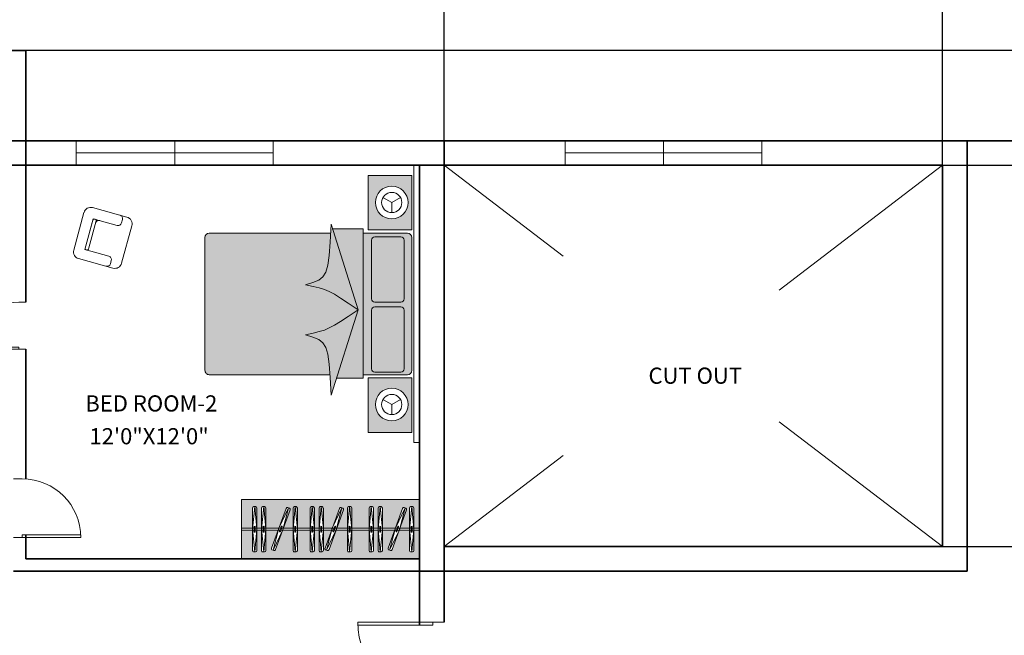
# Model space of a CAD drawing. Units: millimetres. Extents: x 27017497 to 27018854, y 7058029 to 7059154.
# Tile 60 of 91: x 27017886 to 27018246, y 7058409 to 7058634. Entities that reach past the tile are written whole.
import ezdxf

# ---------------------------------------------------------------- set-up
doc = ezdxf.new("R2010")
doc.units = ezdxf.units.MM
for name, color, linetype, lineweight in [('A-ANNO-DIMS', 2, 'Continuous', 18), ('A-AREA-IDEN', 7, 'Continuous', 18), ('A-DOOR', 4, 'Continuous', 20), ('A-FLOR-CASE', 8, 'Continuous', 20), ('A-FLOR-CASE-PATT', 44, 'Continuous', 13), ('A-FLOR-OPEN', 9, 'Continuous', 13), ('A-FURN', 8, 'Continuous', 18), ('A-GLAZ', 4, 'Continuous', 18), ('A-WALL', 7, 'Continuous', 35)]:
    doc.layers.add(name, color=color, linetype=linetype, lineweight=lineweight)
doc.layers.add('A-FURN-PATT', color=177, linetype='Continuous', lineweight=13, true_color=0x293189)
doc.styles.get("Standard").update_dxf_attribs({"font": 'arial.ttf'})
doc.dimstyles.get("Standard").update_dxf_attribs({"dimtxt": 0.18, "dimasz": 0.18, "dimexe": 0.18, "dimexo": 0.0625, "dimgap": 0.09, "dimtad": 0, "dimtih": 1, "dimtoh": 1, "dimdec": 4, "dimzin": 0, "dimdsep": 46, "dimtxsty": 'Standard', "dimcen": 0.09, "dimadec": 0, "dimazin": 0, "dimtfac": 1, "dimtdec": 4, "dimtofl": 0, "dimtmove": 0, "dimatfit": 3, "dimfxl": 1, "dimtolj": 1, "dimtzin": 0, "dimarcsym": 0})

# ---------------------------------------------------------------- blocks, each defined once
blk = doc.blocks.new('CAMMAT')
for p, q in [((1.2731, 0), (-1.2731, 0)), ((1.2731, 0), (1.2731, -0.05)), ((-1.2731, 0), (-1.2731, -0.05)), ((1.2731, -0.05), (-1.2731, -0.05)), ((-1.18, -0.07), (-1.18, -0.47)), ((-1.18, -0.07), (-0.68, -0.07)), ((-0.68, -0.07), (-0.68, -0.47)), ((0.61, -0.07), (-0.61, -0.07)), ((0.68, -0.07), (0.68, -0.47)), ((0.68, -0.07), (1.18, -0.07)), ((1.18, -0.07), (1.18, -0.47)), ((-0.931, -0.2541), (-0.9775, -0.1737)), ((-0.65, -0.11), (-0.65, -0.5169)), ((-0.6152, -0.1695), (-0.6152, -0.4095)), ((-0.0465, -0.1395), (-0.5852, -0.1395)), ((-0.0165, -0.1695), (-0.0165, -0.4095)), ((0.0274, -0.1695), (0.0274, -0.4095)), ((0.5962, -0.1395), (0.0574, -0.1395)), ((0.6262, -0.1695), (0.6262, -0.4095)), ((0.65, -0.11), (0.65, -0.5169)), ((0.9242, -0.2541), (0.8777, -0.1737)), ((-0.931, -0.2541), (-0.9775, -0.3346)), ((-0.931, -0.2541), (-0.8381, -0.2541)), ((0.9242, -0.2541), (0.8777, -0.3346)), ((0.9242, -0.2541), (1.0171, -0.2541)), ((-0.0465, -0.4395), (-0.5852, -0.4395)), ((0.5962, -0.4395), (0.0574, -0.4395)), ((-1.18, -0.47), (-0.68, -0.47)), ((-0.6904, -0.5169), (-0.6904, -0.8)), ((-0.6904, -0.5169), (0.6826, -0.5169)), ((0.68, -0.47), (1.18, -0.47)), ((0.6826, -0.5169), (0.6826, -0.7603)), ((0.0535, -0.5623), (-0.7312, -0.8093)), ((0.0535, -0.5623), (0.8382, -0.8093)), ((-0.65, -0.8139), (-0.65, -1.93)), ((0.65, -0.8204), (0.65, -1.93)), ((0.61, -1.97), (-0.61, -1.97))]:
    blk.add_line(p, q)
for points in [[(-0.1761, -1.0476), (-0.161, -0.9772), (-0.1474, -0.921), (-0.1326, -0.8732), (-0.1139, -0.8282), (-0.0886, -0.7803), (-0.0541, -0.7238), (-0.0076, -0.653), (0.0535, -0.5623)], [(0.2832, -1.0476), (0.2681, -0.9772), (0.2545, -0.921), (0.2396, -0.8732), (0.2209, -0.8282), (0.1957, -0.7803), (0.1611, -0.7238), (0.1147, -0.653), (0.0535, -0.5623)], [(-0.7312, -0.8093), (-0.5683, -0.8185), (-0.4451, -0.828), (-0.3552, -0.8406), (-0.2919, -0.8591), (-0.2489, -0.8862), (-0.2196, -0.9248), (-0.1975, -0.9777), (-0.1761, -1.0476)], [(0.8382, -0.8093), (0.6753, -0.8185), (0.5522, -0.828), (0.4622, -0.8406), (0.399, -0.8591), (0.356, -0.8862), (0.3267, -0.9248), (0.3046, -0.9777), (0.2832, -1.0476)]]:
    blk.add_lwpolyline(points)
for centre, radius in [((-0.931, -0.2541), 0.15), ((-0.931, -0.2541), 0.0929), ((0.9242, -0.2541), 0.15), ((0.9242, -0.2541), 0.0929)]:
    blk.add_circle(centre, radius)
for centre, radius, start, end in [((-0.61, -0.11), 0.04, 90, 180), ((0.61, -0.11), 0.04, 0, 90), ((-0.5852, -0.1695), 0.03, 90, 180), ((-0.0465, -0.1695), 0.03, 360, 90), ((0.0574, -0.1695), 0.03, 90, 180), ((0.5962, -0.1695), 0.03, 360, 90), ((-0.5852, -0.4095), 0.03, 180, 270), ((-0.0465, -0.4095), 0.03, 270, 360), ((0.0574, -0.4095), 0.03, 180, 270), ((0.5962, -0.4095), 0.03, 270, 360), ((-0.61, -1.93), 0.04, 180, 270), ((0.61, -1.93), 0.04, 270, 360)]:
    blk.add_arc(centre, radius, start, end)
blk = doc.blocks.new('*U2')
for p, q in [((0, 0), (0, -6)), ((40, 0), (40, -6))]:
    blk.add_line(p, q)
blk.add_lwpolyline([(0, 0), (0, 40), (1.75, 40), (1.75, 0)], close=True)
blk.add_arc((0, 0), 40, 0, 90)
blk = doc.blocks.new('CHAIR-OCCASIONAL')
for p, q in [((19.6, 18.74), (7.02, 22.21)), ((3.87, 20.42), (0.09, 6.71)), ((4.13, 6.92), (7.23, 18.17)), ((5.25, 10.97), (7.23, 18.17)), ((16.06, 15.73), (7.23, 18.17)), ((7.23, 18.17), (16.06, 15.73)), ((7.23, 18.17), (16.06, 15.73)), ((7.73, 18.03), (7.97, 17.97)), ((7.73, 18.03), (7.97, 17.97)), ((5.25, 10.97), (7.1, 17.68)), ((8.33, 17.34), (5.63, 7.52)), ((17.6, 1.88), (21.39, 15.6)), ((17.64, 16.63), (17.98, 17.86)), ((17.64, 16.63), (17.98, 17.86)), ((5.63, 7.52), (5.5, 7.07)), ((12.96, 4.48), (4.13, 6.92)), ((4.87, 6.71), (4.63, 6.78)), ((1.88, 3.56), (14.46, 0.09)), ((13.86, 2.91), (13.52, 1.68))]:
    blk.add_line(p, q)
for centre, radius, start, end in [((6.34, 19.74), 2.56, 74.5879, 164.5879), ((7.59, 17.54), 0.512, 74.5879, 164.5879), ((16.74, 18.2), 1.28, 344.5879, 74.5879), ((16.74, 18.2), 1.28, 344.5879, 74.5879), ((18.92, 16.28), 2.56, 344.5879, 74.5879), ((7.84, 17.47), 0.512, 344.5879, 74.5879), ((9.36, 16.26), 1.28, 74.5879, 164.5879), ((16.4, 16.97), 1.28, 254.5879, 344.5879), ((16.4, 16.97), 1.28, 254.5879, 344.5879), ((4.76, 7.28), 0.512, 164.5879, 254.5879), ((2.56, 6.03), 2.56, 164.5879, 254.5879), ((5.01, 7.21), 0.512, 254.5879, 344.5879), ((12.62, 3.25), 1.28, 344.5879, 74.5879), ((12.28, 2.02), 1.28, 254.5879, 344.5879), ((15.14, 2.56), 2.56, 254.5879, 344.5879)]:
    blk.add_arc(centre, radius, start, end)
blk = doc.blocks.new('WARDROBE-HANGING')
for p, q in [((0, 21.74), (65.21, 21.74)), ((0, 0), (0, 21.74)), ((65.21, 0), (65.21, 21.74)), ((4.86, 19.15), (4.08, 10.88)), ((4.08, 18.62), (4.08, 3.13)), ((5.18, 19.15), (4.55, 19.15)), ((4.86, 19.15), (5.64, 10.88)), ((5.64, 18.62), (5.64, 3.13)), ((8.14, 19.15), (7.35, 10.88)), ((7.35, 18.62), (7.35, 3.13)), ((8.45, 19.15), (7.82, 19.15)), ((8.14, 19.15), (8.92, 10.88)), ((8.92, 18.62), (8.92, 3.13)), ((16.33, 18.5), (11.03, 3.94)), ((17.25, 18.73), (13.68, 11.22)), ((17.25, 18.73), (15.15, 10.68)), ((17.54, 18.62), (16.95, 18.83)), ((19.66, 19.15), (18.88, 10.88)), ((18.88, 18.62), (18.88, 3.13)), ((19.98, 19.15), (19.35, 19.15)), ((19.66, 19.15), (20.45, 10.88)), ((20.45, 18.62), (20.45, 3.13)), ((25.9, 19.15), (25.12, 10.88)), ((25.12, 18.62), (25.12, 3.13)), ((26.21, 19.15), (25.59, 19.15)), ((25.9, 19.15), (26.68, 10.88)), ((26.68, 18.62), (26.68, 3.13)), ((29.17, 19.15), (28.39, 10.88)), ((28.39, 18.62), (28.39, 3.13)), ((29.49, 19.15), (28.86, 19.15)), ((29.17, 19.15), (29.96, 10.88)), ((29.96, 18.62), (29.96, 3.13)), ((35.87, 18.5), (30.57, 3.94)), ((36.78, 18.73), (33.22, 11.22)), ((36.78, 18.73), (34.69, 10.68)), ((37.08, 18.62), (36.49, 18.83)), ((39.59, 19.15), (38.81, 10.88)), ((38.81, 18.62), (38.81, 3.13)), ((39.9, 19.15), (39.28, 19.15)), ((39.59, 19.15), (40.37, 10.88)), ((40.37, 18.62), (40.37, 3.13)), ((47.49, 19.15), (46.71, 10.88)), ((46.71, 18.62), (46.71, 3.13)), ((47.81, 19.15), (47.18, 19.15)), ((47.49, 19.15), (48.28, 10.88)), ((48.28, 18.62), (48.28, 3.13)), ((50.77, 19.15), (49.98, 10.88)), ((49.98, 18.62), (49.98, 3.13)), ((51.08, 19.15), (50.45, 19.15)), ((50.77, 19.15), (51.55, 10.88)), ((51.55, 18.62), (51.55, 3.13)), ((58.96, 18.5), (53.66, 3.94)), ((59.88, 18.73), (56.31, 11.22)), ((59.88, 18.73), (57.78, 10.68)), ((60.17, 18.62), (59.58, 18.83)), ((62.29, 19.15), (61.51, 10.88)), ((61.51, 18.62), (61.51, 3.13)), ((62.61, 19.15), (61.98, 19.15)), ((62.29, 19.15), (63.08, 10.88)), ((63.08, 18.62), (63.08, 3.13)), ((17.8, 17.96), (12.5, 3.4)), ((37.34, 17.96), (32.04, 3.4)), ((60.43, 17.96), (55.13, 3.4)), ((0, 11.23), (65.21, 11.23)), ((4.86, 2.6), (4.08, 10.88)), ((4.71, 11.83), (4.71, 9.93)), ((4.92, 11.93), (4.8, 11.93)), ((4.86, 2.6), (5.64, 10.88)), ((5.02, 11.83), (5.02, 9.93)), ((8.14, 2.6), (7.35, 10.88)), ((7.98, 11.83), (7.98, 9.93)), ((8.2, 11.93), (8.07, 11.93)), ((8.14, 2.6), (8.92, 10.88)), ((8.29, 11.83), (8.29, 9.93)), ((11.59, 3.17), (13.68, 11.22)), ((14.59, 11.9), (13.94, 10.11)), ((14.89, 11.79), (14.24, 10)), ((14.84, 11.92), (14.72, 11.96)), ((19.66, 2.6), (18.88, 10.88)), ((19.51, 11.83), (19.51, 9.93)), ((19.73, 11.93), (19.6, 11.93)), ((19.66, 2.6), (20.45, 10.88)), ((19.82, 11.83), (19.82, 9.93)), ((25.9, 2.6), (25.12, 10.88)), ((25.74, 11.83), (25.74, 9.93)), ((25.96, 11.93), (25.84, 11.93)), ((25.9, 2.6), (26.68, 10.88)), ((26.06, 11.83), (26.06, 9.93)), ((29.17, 2.6), (28.39, 10.88)), ((29.02, 11.83), (29.02, 9.93)), ((29.24, 11.93), (29.11, 11.93)), ((29.17, 2.6), (29.96, 10.88)), ((29.33, 11.83), (29.33, 9.93)), ((31.12, 3.17), (33.22, 11.22)), ((34.13, 11.9), (33.48, 10.11)), ((34.42, 11.79), (33.77, 10)), ((34.37, 11.92), (34.25, 11.96)), ((39.59, 2.6), (38.81, 10.88)), ((39.43, 11.83), (39.43, 9.93)), ((39.65, 11.93), (39.53, 11.93)), ((39.59, 2.6), (40.37, 10.88)), ((39.75, 11.83), (39.75, 9.93)), ((47.49, 2.6), (46.71, 10.88)), ((47.34, 11.83), (47.34, 9.93)), ((47.56, 11.93), (47.43, 11.93)), ((47.49, 2.6), (48.28, 10.88)), ((47.65, 11.83), (47.65, 9.93)), ((50.77, 2.6), (49.98, 10.88)), ((50.61, 11.83), (50.61, 9.93)), ((50.83, 11.93), (50.7, 11.93)), ((50.77, 2.6), (51.55, 10.88)), ((50.92, 11.83), (50.92, 9.93)), ((54.22, 3.17), (56.31, 11.22)), ((57.22, 11.9), (56.57, 10.11)), ((57.52, 11.79), (56.87, 10)), ((57.47, 11.92), (57.35, 11.96)), ((62.29, 2.6), (61.51, 10.88)), ((62.14, 11.83), (62.14, 9.93)), ((62.36, 11.93), (62.23, 11.93)), ((62.29, 2.6), (63.08, 10.88)), ((62.45, 11.83), (62.45, 9.93)), ((0, 10.51), (65.21, 10.51)), ((4.92, 9.82), (4.8, 9.82)), ((8.2, 9.82), (8.07, 9.82)), ((11.59, 3.17), (15.15, 10.68)), ((14.11, 9.94), (14, 9.98)), ((19.73, 9.82), (19.6, 9.82)), ((25.96, 9.82), (25.84, 9.82)), ((29.24, 9.82), (29.11, 9.82)), ((31.12, 3.17), (34.69, 10.68)), ((33.65, 9.94), (33.53, 9.98)), ((39.65, 9.82), (39.53, 9.82)), ((47.56, 9.82), (47.43, 9.82)), ((50.83, 9.82), (50.7, 9.82)), ((54.22, 3.17), (57.78, 10.68)), ((56.74, 9.94), (56.63, 9.98)), ((62.36, 9.82), (62.23, 9.82)), ((5.18, 2.6), (4.55, 2.6)), ((8.45, 2.6), (7.82, 2.6)), ((11.88, 3.07), (11.29, 3.28)), ((19.98, 2.6), (19.35, 2.6)), ((26.21, 2.6), (25.59, 2.6)), ((29.49, 2.6), (28.86, 2.6)), ((31.42, 3.07), (30.83, 3.28)), ((39.9, 2.6), (39.28, 2.6)), ((47.81, 2.6), (47.18, 2.6)), ((51.08, 2.6), (50.45, 2.6)), ((54.51, 3.07), (53.92, 3.28)), ((62.61, 2.6), (61.98, 2.6)), ((0, 0), (65.21, 0))]:
    blk.add_line(p, q)
for centre, major_axis, start_param, end_param in [((4.55, 18.62), (0, 0.528), 0, 1.570796), ((5.18, 18.62), (0, 0.528), 4.712389, 6.283185), ((7.82, 18.62), (0, 0.528), 0, 1.570796), ((8.45, 18.62), (0, 0.528), 4.712389, 6.283185), ((16.77, 18.34), (0.181, 0.496), 0, 1.570796), ((17.36, 18.12), (0.181, 0.496), -1.570796, 0), ((19.35, 18.62), (0, 0.528), 0, 1.570796), ((19.98, 18.62), (0, 0.528), 4.712389, 6.283185), ((25.59, 18.62), (0, 0.528), 0, 1.570796), ((26.21, 18.62), (0, 0.528), 4.712389, 6.283185), ((28.86, 18.62), (0, 0.528), 0, 1.570796), ((29.49, 18.62), (0, 0.528), 4.712389, 6.283185), ((36.31, 18.34), (0.181, 0.496), 0, 1.570796), ((36.9, 18.12), (0.181, 0.496), -1.570796, 0), ((39.28, 18.62), (0, 0.528), 0, 1.570796), ((39.9, 18.62), (0, 0.528), 4.712389, 6.283185), ((47.18, 18.62), (0, 0.528), 0, 1.570796), ((47.81, 18.62), (0, 0.528), 4.712389, 6.283185), ((50.45, 18.62), (0, 0.528), 0, 1.570796), ((51.08, 18.62), (0, 0.528), 4.712389, 6.283185), ((59.4, 18.34), (0.181, 0.496), 0, 1.570796), ((59.99, 18.12), (0.181, 0.496), -1.570796, 0), ((61.98, 18.62), (0, 0.528), 0, 1.570796), ((62.61, 18.62), (0, 0.528), 4.712389, 6.283185), ((4.8, 11.83), (0, 0.106), 0, 1.570796), ((4.92, 11.83), (0, 0.106), -1.570796, 0), ((8.07, 11.83), (0, 0.106), 0, 1.570796), ((8.2, 11.83), (0, 0.106), -1.570796, 0), ((14.68, 11.86), (0.0361, 0.0993), 0, 1.570796), ((14.8, 11.82), (0.0361, 0.0993), 4.712389, 6.283185), ((19.6, 11.83), (0, 0.106), 0, 1.570796), ((19.73, 11.83), (0, 0.106), -1.570796, 0), ((25.84, 11.83), (0, 0.106), 0, 1.570796), ((25.96, 11.83), (0, 0.106), -1.570796, 0), ((29.11, 11.83), (0, 0.106), 0, 1.570796), ((29.24, 11.83), (0, 0.106), -1.570796, 0), ((34.22, 11.86), (0.0361, 0.0993), 0, 1.570796), ((34.34, 11.82), (0.0361, 0.0993), 4.712389, 6.283185), ((39.53, 11.83), (0, 0.106), 0, 1.570796), ((39.65, 11.83), (0, 0.106), -1.570796, 0), ((47.43, 11.83), (0, 0.106), 0, 1.570796), ((47.56, 11.83), (0, 0.106), -1.570796, 0), ((50.7, 11.83), (0, 0.106), 0, 1.570796), ((50.83, 11.83), (0, 0.106), -1.570796, 0), ((57.31, 11.86), (0.0361, 0.0993), 0, 1.570796), ((57.43, 11.82), (0.0361, 0.0993), 4.712389, 6.283185), ((62.23, 11.83), (0, 0.106), 0, 1.570796), ((62.36, 11.83), (0, 0.106), -1.570796, 0), ((4.8, 9.93), (0, 0.106), 1.570796, 3.141593), ((4.92, 9.93), (0, 0.106), 3.141593, 4.712389), ((8.07, 9.93), (0, 0.106), 1.570796, 3.141593), ((8.2, 9.93), (0, 0.106), 3.141593, 4.712389), ((14.03, 10.08), (0.0361, 0.0993), 1.570796, 3.141593), ((14.15, 10.03), (0.0361, 0.0993), 3.141593, 4.712389), ((19.6, 9.93), (0, 0.106), 1.570796, 3.141593), ((19.73, 9.93), (0, 0.106), 3.141593, 4.712389), ((25.84, 9.93), (0, 0.106), 1.570796, 3.141593), ((25.96, 9.93), (0, 0.106), 3.141593, 4.712389), ((29.11, 9.93), (0, 0.106), 1.570796, 3.141593), ((29.24, 9.93), (0, 0.106), 3.141593, 4.712389), ((33.57, 10.08), (0.0361, 0.0993), 1.570796, 3.141593), ((33.69, 10.03), (0.0361, 0.0993), 3.141593, 4.712389), ((39.53, 9.93), (0, 0.106), 1.570796, 3.141593), ((39.65, 9.93), (0, 0.106), 3.141593, 4.712389), ((47.43, 9.93), (0, 0.106), 1.570796, 3.141593), ((47.56, 9.93), (0, 0.106), 3.141593, 4.712389), ((50.7, 9.93), (0, 0.106), 1.570796, 3.141593), ((50.83, 9.93), (0, 0.106), 3.141593, 4.712389), ((56.66, 10.08), (0.0361, 0.0993), 1.570796, 3.141593), ((56.78, 10.03), (0.0361, 0.0993), 3.141593, 4.712389), ((62.23, 9.93), (0, 0.106), 1.570796, 3.141593), ((62.36, 9.93), (0, 0.106), 3.141593, 4.712389), ((11.47, 3.78), (0.181, 0.496), 1.570796, 3.141593), ((31.01, 3.78), (0.181, 0.496), 1.570796, 3.141593), ((54.1, 3.78), (0.181, 0.496), 1.570796, 3.141593), ((4.55, 3.13), (0, 0.528), 1.570796, 3.141593), ((5.18, 3.13), (0, 0.528), 3.141593, 4.712389), ((7.82, 3.13), (0, 0.528), 1.570796, 3.141593), ((8.45, 3.13), (0, 0.528), 3.141593, 4.712389), ((12.06, 3.56), (0.181, 0.496), 3.141593, 4.712389), ((19.35, 3.13), (0, 0.528), 1.570796, 3.141593), ((19.98, 3.13), (0, 0.528), 3.141593, 4.712389), ((25.59, 3.13), (0, 0.528), 1.570796, 3.141593), ((26.21, 3.13), (0, 0.528), 3.141593, 4.712389), ((28.86, 3.13), (0, 0.528), 1.570796, 3.141593), ((29.49, 3.13), (0, 0.528), 3.141593, 4.712389), ((31.6, 3.56), (0.181, 0.496), 3.141593, 4.712389), ((39.28, 3.13), (0, 0.528), 1.570796, 3.141593), ((39.9, 3.13), (0, 0.528), 3.141593, 4.712389), ((47.18, 3.13), (0, 0.528), 1.570796, 3.141593), ((47.81, 3.13), (0, 0.528), 3.141593, 4.712389), ((50.45, 3.13), (0, 0.528), 1.570796, 3.141593), ((51.08, 3.13), (0, 0.528), 3.141593, 4.712389), ((54.69, 3.56), (0.181, 0.496), 3.141593, 4.712389), ((61.98, 3.13), (0, 0.528), 1.570796, 3.141593), ((62.61, 3.13), (0, 0.528), 3.141593, 4.712389)]:
    blk.add_ellipse(centre, major_axis=major_axis, ratio=0.888892, start_param=start_param, end_param=end_param)
blk = doc.blocks.new('WINDOW-SINGLE-LIGHT')
blk.add_lwpolyline([(36, 4.5), (36, 0), (0, 0), (0, 9), (36, 9), (36, 4.5), (0, 4.5)])
blk = doc.blocks.new('*D48')
at = {"layer": 'A-ANNO-DIMS', "color": 0, "lineweight": -2, "transparency": 16777216}
for p, q in [((27018463.5, 7058622.91), (27017497.54, 7058622.91)), ((27017497.72, 7058622.73), (27017497.72, 7058357.75)), ((27017497.72, 7058092.41), (27017497.72, 7058357.39)), ((27018555.13, 7058092.23), (27017497.54, 7058092.23))]:
    blk.add_line(p, q, dxfattribs=at)
at = {"layer": 'A-ANNO-DIMS', "color": 0, "transparency": 16777216}
for points in [[(27017497.69, 7058622.73), (27017497.75, 7058622.73), (27017497.72, 7058622.91)], [(27017497.69, 7058092.41), (27017497.75, 7058092.41), (27017497.72, 7058092.23)]]:
    blk.add_solid(points, dxfattribs=at)
at = {"layer": 'Defpoints', "color": 0, "transparency": 16777216}
for p in [(27018463.56, 7058622.91), (27017497.72, 7058092.23), (27018555.19, 7058092.23)]:
    blk.add_point(p, dxfattribs=at)
at = {"layer": 'A-ANNO-DIMS', "color": 0, "transparency": 16777216, "insert": (27017497.72, 7058357.57), "char_height": 0.18, "attachment_point": 5}
blk.add_mtext('\\A1;530.7', dxfattribs=at)
blk = doc.blocks.new('*D49')
at = {"layer": 'A-ANNO-DIMS', "color": 0, "lineweight": -2, "transparency": 16777216}
for p, q in [((27018041.17, 7058580.97), (27018041.17, 7058686.54)), ((27018041.35, 7058686.36), (27018131.93, 7058686.36)), ((27018223.43, 7058686.36), (27018132.84, 7058686.36)), ((27018223.61, 7058580.97), (27018223.61, 7058686.54))]:
    blk.add_line(p, q, dxfattribs=at)
at = {"layer": 'A-ANNO-DIMS', "color": 0, "transparency": 16777216}
for points in [[(27018041.35, 7058686.39), (27018041.35, 7058686.33), (27018041.17, 7058686.36)], [(27018223.43, 7058686.39), (27018223.43, 7058686.33), (27018223.61, 7058686.36)]]:
    blk.add_solid(points, dxfattribs=at)
at = {"layer": 'Defpoints', "color": 0, "transparency": 16777216}
for p in [(27018223.61, 7058686.36), (27018041.17, 7058580.91), (27018223.61, 7058580.91)]:
    blk.add_point(p, dxfattribs=at)
at = {"layer": 'A-ANNO-DIMS', "color": 0, "transparency": 16777216, "insert": (27018132.39, 7058686.36), "char_height": 0.18, "attachment_point": 5}
blk.add_mtext('\\A1;182.44', dxfattribs=at)
blk = doc.blocks.new('*D50')
at = {"layer": 'A-ANNO-DIMS', "color": 0, "lineweight": -2, "transparency": 16777216}
for p, q in [((27018223.67, 7058580.91), (27018854.24, 7058580.91)), ((27018854.06, 7058580.73), (27018854.06, 7058511.34)), ((27018854.06, 7058441.59), (27018854.06, 7058510.98)), ((27018223.67, 7058441.41), (27018854.24, 7058441.41))]:
    blk.add_line(p, q, dxfattribs=at)
at = {"layer": 'A-ANNO-DIMS', "color": 0, "transparency": 16777216}
for points in [[(27018854.03, 7058580.73), (27018854.09, 7058580.73), (27018854.06, 7058580.91)], [(27018854.03, 7058441.59), (27018854.09, 7058441.59), (27018854.06, 7058441.41)]]:
    blk.add_solid(points, dxfattribs=at)
at = {"layer": 'Defpoints', "color": 0, "transparency": 16777216}
for p in [(27018223.61, 7058580.91), (27018223.61, 7058441.41), (27018854.06, 7058441.41)]:
    blk.add_point(p, dxfattribs=at)
at = {"layer": 'A-ANNO-DIMS', "color": 0, "transparency": 16777216, "insert": (27018854.06, 7058511.16), "char_height": 0.18, "attachment_point": 5}
blk.add_mtext('\\A1;139.5', dxfattribs=at)

msp = doc.modelspace()

# ---------------------------------------------------------------- hatches: boundary and pattern name
at = {"layer": 'A-FLOR-CASE-PATT'}
h = msp.add_hatch(color=256, dxfattribs=at)
h.dxf.hatch_style = 1
edge = h.paths.add_edge_path()
edge.add_ellipse((27017983.826, 7058455.241), major_axis=(0.181, 0.496), ratio=0.8888917, start_angle=0, end_angle=90, ccw=False)
edge.add_line((27017984.007, 7058455.738), (27017984.301, 7058455.631))
edge.add_line((27017984.301, 7058455.631), (27017982.349, 7058448.136))
edge.add_line((27017982.349, 7058448.136), (27017985.935, 7058448.136))
edge.add_line((27017985.935, 7058448.136), (27017985.935, 7058455.723))
edge.add_ellipse((27017986.405, 7058455.529), major_axis=(0, 0.528), ratio=0.8888917, start_angle=0, end_angle=90, ccw=False)
edge.add_line((27017986.405, 7058456.058), (27017986.718, 7058456.058))
edge.add_line((27017986.718, 7058456.058), (27017987.467, 7058448.136))
edge.add_line((27017987.467, 7058448.136), (27017992.173, 7058448.136))
edge.add_line((27017992.173, 7058448.136), (27017992.173, 7058455.723))
edge.add_ellipse((27017992.642, 7058455.529), major_axis=(0, 0.528), ratio=0.8888917, start_angle=0, end_angle=90, ccw=False)
edge.add_line((27017992.642, 7058456.058), (27017992.955, 7058456.058))
edge.add_line((27017992.955, 7058456.058), (27017993.704, 7058448.136))
edge.add_line((27017993.704, 7058448.136), (27017995.446, 7058448.136))
edge.add_line((27017995.446, 7058448.136), (27017995.446, 7058455.723))
edge.add_ellipse((27017995.915, 7058455.529), major_axis=(0, 0.528), ratio=0.8888917, start_angle=0, end_angle=90, ccw=False)
edge.add_line((27017995.915, 7058456.058), (27017996.228, 7058456.058))
edge.add_line((27017996.228, 7058456.058), (27017996.978, 7058448.136))
edge.add_line((27017996.978, 7058448.136), (27018000.277, 7058448.136))
edge.add_line((27018000.277, 7058448.136), (27018002.988, 7058455.584))
edge.add_ellipse((27018003.363, 7058455.241), major_axis=(0.181, 0.496), ratio=0.8888917, start_angle=0, end_angle=90, ccw=False)
edge.add_line((27018003.543, 7058455.738), (27018003.838, 7058455.631))
edge.add_line((27018003.838, 7058455.631), (27018001.886, 7058448.136))
edge.add_line((27018001.886, 7058448.136), (27018005.861, 7058448.136))
edge.add_line((27018005.861, 7058448.136), (27018005.861, 7058455.723))
edge.add_ellipse((27018006.331, 7058455.529), major_axis=(0, 0.528), ratio=0.8888917, start_angle=0, end_angle=90, ccw=False)
edge.add_line((27018006.331, 7058456.058), (27018006.644, 7058456.058))
edge.add_line((27018006.644, 7058456.058), (27018007.393, 7058448.136))
edge.add_line((27018007.393, 7058448.136), (27018013.765, 7058448.136))
edge.add_line((27018013.765, 7058448.136), (27018013.765, 7058455.723))
edge.add_ellipse((27018014.235, 7058455.529), major_axis=(0, 0.528), ratio=0.8888917, start_angle=0, end_angle=90, ccw=False)
edge.add_line((27018014.235, 7058456.058), (27018015.033, 7058456.058))
edge.add_ellipse((27018014.861, 7058455.529), major_axis=(0, 0.528), ratio=0.8888917, start_angle=270, end_angle=360, ccw=False)
edge.add_line((27018015.331, 7058455.529), (27018015.331, 7058448.136))
edge.add_line((27018015.331, 7058448.136), (27018017.039, 7058448.136))
edge.add_line((27018017.039, 7058448.136), (27018017.039, 7058455.723))
edge.add_ellipse((27018017.508, 7058455.529), major_axis=(0, 0.528), ratio=0.8888917, start_angle=0, end_angle=90, ccw=False)
edge.add_line((27018017.508, 7058456.058), (27018018.306, 7058456.058))
edge.add_ellipse((27018018.134, 7058455.529), major_axis=(0, 0.528), ratio=0.8888917, start_angle=270, end_angle=360, ccw=False)
edge.add_line((27018018.604, 7058455.529), (27018018.604, 7058448.136))
edge.add_line((27018018.604, 7058448.136), (27018023.371, 7058448.136))
edge.add_line((27018023.371, 7058448.136), (27018026.082, 7058455.584))
edge.add_ellipse((27018026.457, 7058455.241), major_axis=(0.181, 0.496), ratio=0.8888917, start_angle=0, end_angle=90, ccw=False)
edge.add_line((27018026.637, 7058455.738), (27018026.932, 7058455.631))
edge.add_line((27018026.932, 7058455.631), (27018024.98, 7058448.136))
edge.add_line((27018024.98, 7058448.136), (27018028.566, 7058448.136))
edge.add_line((27018028.566, 7058448.136), (27018028.566, 7058455.723))
edge.add_ellipse((27018029.035, 7058455.529), major_axis=(0, 0.528), ratio=0.8888917, start_angle=0, end_angle=90, ccw=False)
edge.add_line((27018029.035, 7058456.058), (27018029.833, 7058456.058))
edge.add_ellipse((27018029.661, 7058455.529), major_axis=(0, 0.528), ratio=0.8888917, start_angle=270, end_angle=360, ccw=False)
edge.add_line((27018030.131, 7058455.529), (27018030.131, 7058448.136))
edge.add_line((27018030.131, 7058448.136), (27018032.166, 7058448.136))
edge.add_line((27018032.166, 7058448.136), (27018032.166, 7058458.642))
edge.add_line((27018032.166, 7058458.642), (27017967.055, 7058458.642))
edge.add_line((27017967.055, 7058458.642), (27017967.055, 7058448.136))
edge.add_line((27017967.055, 7058448.136), (27017971.135, 7058448.136))
edge.add_line((27017971.135, 7058448.136), (27017971.135, 7058455.723))
edge.add_ellipse((27017971.604, 7058455.529), major_axis=(0, 0.528), ratio=0.8888917, start_angle=0, end_angle=90, ccw=False)
edge.add_line((27017971.604, 7058456.058), (27017971.917, 7058456.058))
edge.add_line((27017971.917, 7058456.058), (27017972.666, 7058448.136))
edge.add_line((27017972.666, 7058448.136), (27017974.408, 7058448.136))
edge.add_line((27017974.408, 7058448.136), (27017974.408, 7058455.723))
edge.add_ellipse((27017974.877, 7058455.529), major_axis=(0, 0.528), ratio=0.8888917, start_angle=0, end_angle=90, ccw=False)
edge.add_line((27017974.877, 7058456.058), (27017975.19, 7058456.058))
edge.add_line((27017975.19, 7058456.058), (27017975.94, 7058448.136))
edge.add_line((27017975.94, 7058448.136), (27017980.74, 7058448.136))
edge.add_line((27017980.74, 7058448.136), (27017983.451, 7058455.584))
edge = h.paths.add_edge_path()
edge.add_line((27017985.935, 7058447.411), (27017982.142, 7058447.411))
edge.add_line((27017982.142, 7058447.411), (27017979.49, 7058440.125))
edge.add_ellipse((27017979.115, 7058440.467), major_axis=(0.181, 0.496), ratio=0.8888917, start_angle=180, end_angle=270, ccw=False)
edge.add_line((27017978.934, 7058439.971), (27017978.185, 7058440.244))
edge.add_ellipse((27017978.527, 7058440.682), major_axis=(0.181, 0.496), ratio=0.8888917, start_angle=90, end_angle=180, ccw=False)
edge.add_line((27017978.086, 7058440.842), (27017980.477, 7058447.411))
edge.add_line((27017980.477, 7058447.411), (27017975.973, 7058447.411))
edge.add_line((27017975.973, 7058447.411), (27017975.973, 7058439.842))
edge.add_ellipse((27017975.503, 7058440.035), major_axis=(0, 0.528), ratio=0.8888917, start_angle=180, end_angle=270, ccw=False)
edge.add_line((27017975.503, 7058439.507), (27017974.706, 7058439.507))
edge.add_ellipse((27017974.877, 7058440.035), major_axis=(0, 0.528), ratio=0.8888917, start_angle=90, end_angle=180, ccw=False)
edge.add_line((27017974.408, 7058440.035), (27017974.408, 7058447.411))
edge.add_line((27017974.408, 7058447.411), (27017972.7, 7058447.411))
edge.add_line((27017972.7, 7058447.411), (27017972.7, 7058439.842))
edge.add_ellipse((27017972.23, 7058440.035), major_axis=(0, 0.528), ratio=0.8888917, start_angle=180, end_angle=270, ccw=False)
edge.add_line((27017972.23, 7058439.507), (27017971.432, 7058439.507))
edge.add_ellipse((27017971.604, 7058440.035), major_axis=(0, 0.528), ratio=0.8888917, start_angle=90, end_angle=180, ccw=False)
edge.add_line((27017971.135, 7058440.035), (27017971.135, 7058447.411))
edge.add_line((27017971.135, 7058447.411), (27017967.055, 7058447.411))
edge.add_line((27017967.055, 7058447.411), (27017967.055, 7058436.912))
edge.add_line((27017967.055, 7058436.912), (27018032.166, 7058436.912))
edge.add_line((27018032.166, 7058436.912), (27018032.166, 7058447.411))
edge.add_line((27018032.166, 7058447.411), (27018030.131, 7058447.411))
edge.add_line((27018030.131, 7058447.411), (27018030.131, 7058439.842))
edge.add_ellipse((27018029.661, 7058440.035), major_axis=(0, 0.528), ratio=0.8888917, start_angle=180, end_angle=270, ccw=False)
edge.add_line((27018029.661, 7058439.507), (27018028.863, 7058439.507))
edge.add_ellipse((27018029.035, 7058440.035), major_axis=(0, 0.528), ratio=0.8888917, start_angle=90, end_angle=180, ccw=False)
edge.add_line((27018028.566, 7058440.035), (27018028.566, 7058447.411))
edge.add_line((27018028.566, 7058447.411), (27018024.773, 7058447.411))
edge.add_line((27018024.773, 7058447.411), (27018022.121, 7058440.125))
edge.add_ellipse((27018021.746, 7058440.467), major_axis=(0.181, 0.496), ratio=0.8888917, start_angle=180, end_angle=270, ccw=False)
edge.add_line((27018021.565, 7058439.971), (27018020.815, 7058440.244))
edge.add_ellipse((27018021.157, 7058440.682), major_axis=(0.181, 0.496), ratio=0.8888917, start_angle=90, end_angle=180, ccw=False)
edge.add_line((27018020.716, 7058440.842), (27018023.107, 7058447.411))
edge.add_line((27018023.107, 7058447.411), (27018018.604, 7058447.411))
edge.add_line((27018018.604, 7058447.411), (27018018.604, 7058439.842))
edge.add_ellipse((27018018.134, 7058440.035), major_axis=(0, 0.528), ratio=0.8888917, start_angle=180, end_angle=270, ccw=False)
edge.add_line((27018018.134, 7058439.507), (27018017.336, 7058439.507))
edge.add_ellipse((27018017.508, 7058440.035), major_axis=(0, 0.528), ratio=0.8888917, start_angle=90, end_angle=180, ccw=False)
edge.add_line((27018017.039, 7058440.035), (27018017.039, 7058447.411))
edge.add_line((27018017.039, 7058447.411), (27018015.331, 7058447.411))
edge.add_line((27018015.331, 7058447.411), (27018015.331, 7058439.842))
edge.add_ellipse((27018014.861, 7058440.035), major_axis=(0, 0.528), ratio=0.8888917, start_angle=180, end_angle=270, ccw=False)
edge.add_line((27018014.861, 7058439.507), (27018014.063, 7058439.507))
edge.add_ellipse((27018014.235, 7058440.035), major_axis=(0, 0.528), ratio=0.8888917, start_angle=90, end_angle=180, ccw=False)
edge.add_line((27018013.765, 7058440.035), (27018013.765, 7058447.411))
edge.add_line((27018013.765, 7058447.411), (27018007.427, 7058447.411))
edge.add_line((27018007.427, 7058447.411), (27018007.427, 7058439.842))
edge.add_ellipse((27018006.957, 7058440.035), major_axis=(0, 0.528), ratio=0.8888917, start_angle=180, end_angle=270, ccw=False)
edge.add_line((27018006.957, 7058439.507), (27018006.159, 7058439.507))
edge.add_ellipse((27018006.331, 7058440.035), major_axis=(0, 0.528), ratio=0.8888917, start_angle=90, end_angle=180, ccw=False)
edge.add_line((27018005.861, 7058440.035), (27018005.861, 7058447.411))
edge.add_line((27018005.861, 7058447.411), (27018001.679, 7058447.411))
edge.add_line((27018001.679, 7058447.411), (27017999.027, 7058440.125))
edge.add_ellipse((27017998.652, 7058440.467), major_axis=(0.181, 0.496), ratio=0.8888917, start_angle=180, end_angle=270, ccw=False)
edge.add_line((27017998.471, 7058439.971), (27017997.721, 7058440.244))
edge.add_ellipse((27017998.063, 7058440.682), major_axis=(0.181, 0.496), ratio=0.8888917, start_angle=90, end_angle=180, ccw=False)
edge.add_line((27017997.622, 7058440.842), (27018000.013, 7058447.411))
edge.add_line((27018000.013, 7058447.411), (27017997.011, 7058447.411))
edge.add_line((27017997.011, 7058447.411), (27017997.011, 7058439.842))
edge.add_ellipse((27017996.541, 7058440.035), major_axis=(0, 0.528), ratio=0.8888917, start_angle=180, end_angle=270, ccw=False)
edge.add_line((27017996.541, 7058439.507), (27017995.744, 7058439.507))
edge.add_ellipse((27017995.915, 7058440.035), major_axis=(0, 0.528), ratio=0.8888917, start_angle=90, end_angle=180, ccw=False)
edge.add_line((27017995.446, 7058440.035), (27017995.446, 7058447.411))
edge.add_line((27017995.446, 7058447.411), (27017993.738, 7058447.411))
edge.add_line((27017993.738, 7058447.411), (27017993.738, 7058439.842))
edge.add_ellipse((27017993.268, 7058440.035), major_axis=(0, 0.528), ratio=0.8888917, start_angle=180, end_angle=270, ccw=False)
edge.add_line((27017993.268, 7058439.507), (27017992.47, 7058439.507))
edge.add_ellipse((27017992.642, 7058440.035), major_axis=(0, 0.528), ratio=0.8888917, start_angle=90, end_angle=180, ccw=False)
edge.add_line((27017992.173, 7058440.035), (27017992.173, 7058447.411))
edge.add_line((27017992.173, 7058447.411), (27017987.5, 7058447.411))
edge.add_line((27017987.5, 7058447.411), (27017987.5, 7058439.842))
edge.add_ellipse((27017987.031, 7058440.035), major_axis=(0, 0.528), ratio=0.8888917, start_angle=180, end_angle=270, ccw=False)
edge.add_line((27017987.031, 7058439.507), (27017986.233, 7058439.507))
edge.add_ellipse((27017986.405, 7058440.035), major_axis=(0, 0.528), ratio=0.8888917, start_angle=90, end_angle=180, ccw=False)
edge.add_line((27017985.935, 7058440.035), (27017985.935, 7058447.411))
at = {"layer": 'A-FURN-PATT'}
h = msp.add_hatch(color=256, dxfattribs=at)
h.dxf.hatch_style = 1
h.paths.add_polyline_path([(27017999.183, 7058534.736), (27017997.391, 7058535.48), (27017995.488, 7058536.07), (27017993.247, 7058536.613), (27017990.443, 7058537.215), (27017993.228, 7058538.068), (27017995.334, 7058538.948), (27017996.872, 7058540.115), (27017997.954, 7058541.828), (27017998.689, 7058544.346), (27017999.191, 7058547.929), (27017999.569, 7058552.834), (27017999.754, 7058556.09), (27017955.298, 7058556.09, 0.4142136), (27017953.705, 7058554.497), (27017953.705, 7058505.904, 0.4142136), (27017955.298, 7058504.311), (27017999.492, 7058504.311), (27017999.191, 7058508.207), (27017998.689, 7058511.79), (27017997.954, 7058514.308), (27017996.872, 7058516.021), (27017995.334, 7058517.188), (27017993.228, 7058518.068), (27017990.443, 7058518.92), (27017993.247, 7058519.523), (27017995.488, 7058520.066), (27017997.391, 7058520.656), (27017999.183, 7058521.4), (27018001.091, 7058522.407), (27018003.341, 7058523.782), (27018006.16, 7058525.633), (27018009.774, 7058528.068), (27018006.16, 7058530.503), (27018003.341, 7058532.354), (27018001.091, 7058533.729)])
h.paths.add_polyline_path([(27018011.581, 7058557.699), (27018000.447, 7058557.699), (27018009.774, 7058528.068), (27018001.888, 7058503.014), (27018011.581, 7058503.014)])
h.paths.add_polyline_path([(27018000.447, 7058557.699), (27017999.844, 7058557.699), (27017999.569, 7058552.834), (27017999.191, 7058547.929), (27017998.689, 7058544.346), (27017997.954, 7058541.828), (27017996.872, 7058540.115), (27017995.334, 7058538.948), (27017993.228, 7058538.068), (27017990.443, 7058537.215), (27017993.247, 7058536.613), (27017995.488, 7058536.07), (27017997.391, 7058535.48), (27017999.183, 7058534.736), (27018001.091, 7058533.729), (27018003.341, 7058532.354), (27018006.16, 7058530.503), (27018009.774, 7058528.068)])
h.paths.add_polyline_path([(27018009.774, 7058528.068), (27018006.16, 7058525.633), (27018003.341, 7058523.782), (27018001.091, 7058522.407), (27017999.183, 7058521.4), (27017997.391, 7058520.656), (27017995.488, 7058520.066), (27017993.247, 7058519.523), (27017990.443, 7058518.92), (27017993.228, 7058518.068), (27017995.334, 7058517.188), (27017996.872, 7058516.021), (27017997.954, 7058514.308), (27017998.689, 7058511.79), (27017999.191, 7058508.207), (27017999.569, 7058503.301), (27017999.936, 7058496.813)])
h.paths.add_polyline_path([(27018029.382, 7058554.497, 0.4142136), (27018027.789, 7058556.09), (27018011.581, 7058556.09), (27018011.581, 7058504.311), (27018027.789, 7058504.311, 0.4142136), (27018029.382, 7058505.904)])
h.paths.add_polyline_path([(27018014.664, 7058553.51, -0.4142136), (27018015.859, 7058554.705), (27018025.419, 7058554.705, -0.4142136), (27018026.613, 7058553.51), (27018026.613, 7058532.051, -0.4142136), (27018025.419, 7058530.856), (27018015.859, 7058530.856, -0.4142136), (27018014.664, 7058532.051)], flags=0)
h.paths.add_polyline_path([(27018015.859, 7058529.109), (27018025.419, 7058529.109, -0.4142136), (27018026.613, 7058527.914), (27018026.613, 7058506.454, -0.4142136), (27018025.419, 7058505.259), (27018015.859, 7058505.259, -0.4142136), (27018014.664, 7058506.454), (27018014.664, 7058527.914, -0.4142136)], flags=16)
h.paths.add_polyline_path([(27018029.382, 7058577.2), (27018013.45, 7058577.2), (27018013.45, 7058557.285), (27018029.382, 7058557.285)])
h.paths.add_polyline_path([(27018016.074, 7058567.284, -1), (27018028.023, 7058567.284, -1)], flags=16)
h.paths.add_polyline_path([(27018018.349, 7058567.284, -1), (27018025.749, 7058567.284, -1)], flags=0)
h.paths.add_polyline_path([(27018029.382, 7058503.116), (27018013.45, 7058503.116), (27018013.45, 7058483.201), (27018029.382, 7058483.201)])
h.paths.add_polyline_path([(27018016.074, 7058493.391, -1), (27018028.023, 7058493.391, -1)], flags=16)
h.paths.add_polyline_path([(27018018.349, 7058493.391, -1), (27018025.749, 7058493.391, -1)], flags=0)
h.paths.add_polyline_path([(27018026.613, 7058553.51, 0.4142136), (27018025.419, 7058554.705), (27018015.859, 7058554.705, 0.4142136), (27018014.664, 7058553.51), (27018014.664, 7058532.051, 0.4142136), (27018015.859, 7058530.856), (27018025.419, 7058530.856, 0.4142136), (27018026.613, 7058532.051)], flags=16)
h = msp.add_hatch(color=256, dxfattribs=at)
h.dxf.hatch_style = 1
h.paths.add_polyline_path([(27018026.613, 7058553.51, 0.4142136), (27018025.419, 7058554.705), (27018015.859, 7058554.705, 0.4142136), (27018014.664, 7058553.51), (27018014.664, 7058532.051, 0.4142136), (27018015.859, 7058530.856), (27018025.419, 7058530.856, 0.4142136), (27018026.613, 7058532.051)])
h.paths.add_polyline_path([(27018026.613, 7058527.914, 0.4142136), (27018025.419, 7058529.109), (27018015.859, 7058529.109, 0.4142136), (27018014.664, 7058527.914), (27018014.664, 7058506.454, 0.4142136), (27018015.859, 7058505.259), (27018025.419, 7058505.259, 0.4142136), (27018026.613, 7058506.454)])

# ---------------------------------------------------------------- linework, layer by layer
at = {"layer": 'A-FLOR-OPEN'}
for p, q in [((27018041.166, 7058580.912), (27018084.715, 7058547.613)), ((27018163.834, 7058535.209), (27018223.606, 7058580.912)), ((27018163.834, 7058487.116), (27018223.606, 7058441.412)), ((27018041.166, 7058441.412), (27018084.715, 7058474.712))]:
    msp.add_line(p, q, dxfattribs=at)
at = {"layer": 'A-WALL'}
for p, q in [((27017777.344, 7058622.912), (27017888.211, 7058622.912)), ((27017888.166, 7058622.912), (27017888.166, 7058530.804)), ((27017613.666, 7058589.912), (27018310.606, 7058589.912)), ((27018041.166, 7058589.912), (27018041.166, 7058413.839)), ((27018232.606, 7058589.912), (27018232.606, 7058432.412)), ((27017622.666, 7058580.912), (27018223.606, 7058580.912)), ((27018032.166, 7058580.912), (27018032.166, 7058412.636)), ((27018223.606, 7058580.912), (27018223.606, 7058441.412)), ((27017888.166, 7058513.597), (27017888.166, 7058466.164)), ((27017888.166, 7058445.749), (27017888.166, 7058436.912)), ((27018041.166, 7058441.412), (27018223.606, 7058441.412)), ((27017888.166, 7058436.912), (27018032.166, 7058436.912)), ((27017883.666, 7058432.412), (27018041.166, 7058432.412)), ((27018041.166, 7058432.412), (27018232.606, 7058432.412))]:
    msp.add_line(p, q, dxfattribs=at)

# ---------------------------------------------------------------- block references
at = {"layer": 'A-DOOR'}
for p, xscale, yscale, zscale, rotation in [((27017885.592, 7058513.597), 0.4301822298564029, 0.4301822298564029, 0.4301822298564029, 90.00000000000003), ((27017886.848, 7058444.814), -0.5347783892510444, 0.5347783892510444, 0.5347783892510444, 270), ((27018037.095, 7058413.839), -0.6870473523349573, 0.6870473523349573, 0.6870473523349573, 90)]:
    msp.add_blockref('*U2', p, dxfattribs=dict(at, xscale=xscale, yscale=yscale, zscale=zscale, rotation=rotation))
at = {"layer": 'A-FLOR-CASE'}
msp.add_blockref('WARDROBE-HANGING', (27017967.055, 7058436.905), dxfattribs=at)
at = {"layer": 'A-FURN', "xscale": 39.82996475819422, "yscale": 39.82996475819422, "zscale": 39.82996475819422, "rotation": 270}
msp.add_blockref('CAMMAT', (27018032.17, 7058530.2), dxfattribs=at)
at = {"layer": 'A-FURN'}
msp.add_blockref('CHAIR-OCCASIONAL', (27017905.575, 7058543.199), dxfattribs=at)
at = {"layer": 'A-GLAZ'}
for p in [(27017906.636, 7058580.927), (27017942.634, 7058580.929), (27018085.438, 7058580.913), (27018121.438, 7058580.913)]:
    msp.add_blockref('WINDOW-SINGLE-LIGHT', p, dxfattribs=at)

# ---------------------------------------------------------------- texts
at = {"layer": 'A-ANNO-DIMS'}
msp.add_text('12\'0"X12\'0"', height=5.91176, dxfattribs=at).set_placement((27017911.452, 7058478.846))
at = {"layer": 'A-AREA-IDEN'}
for s, p in [('CUT OUT', (27018115.979, 7058500.992)), ('BED ROOM-2', (27017909.917, 7058490.843))]:
    msp.add_text(s, height=5.9118, dxfattribs=at).set_placement(p)

# ---------------------------------------------------------------- dimensions: what is measured, and where the dimension line sits
at = {"layer": 'A-ANNO-DIMS'}
dim = msp.add_linear_dim(base=(27018223.606, 7058686.362), p1=(27018041.166, 7058580.912), p2=(27018223.606, 7058580.912), dimstyle='Standard', override={"dimdec": 2, "dimlfac": 1, "dimrnd": 0, "dimzin": 0, "dimdsep": 46, "dimlunit": 2}, dxfattribs=at)
dim.commit()
dim.dimension.update_dxf_attribs({"geometry": '*D49', "text_midpoint": (27018132.386, 7058686.362)})
for base, p1, p2, picture, middle in [((27017497.716, 7058092.23), (27018463.561, 7058622.912), (27018555.192, 7058092.23), '*D48', (27017497.716, 7058357.571)), ((27018854.056, 7058441.412), (27018223.606, 7058580.912), (27018223.606, 7058441.412), '*D50', (27018854.056, 7058511.162))]:
    dim = msp.add_linear_dim(base=base, p1=p1, p2=p2, angle=90, dimstyle='Standard', override={"dimdec": 1, "dimlfac": 1, "dimrnd": 0, "dimzin": 0, "dimdsep": 46, "dimlunit": 2}, dxfattribs=at)
    dim.commit()
    dim.dimension.update_dxf_attribs({"geometry": picture, "text_midpoint": middle})

doc.saveas('drawing.dxf')
